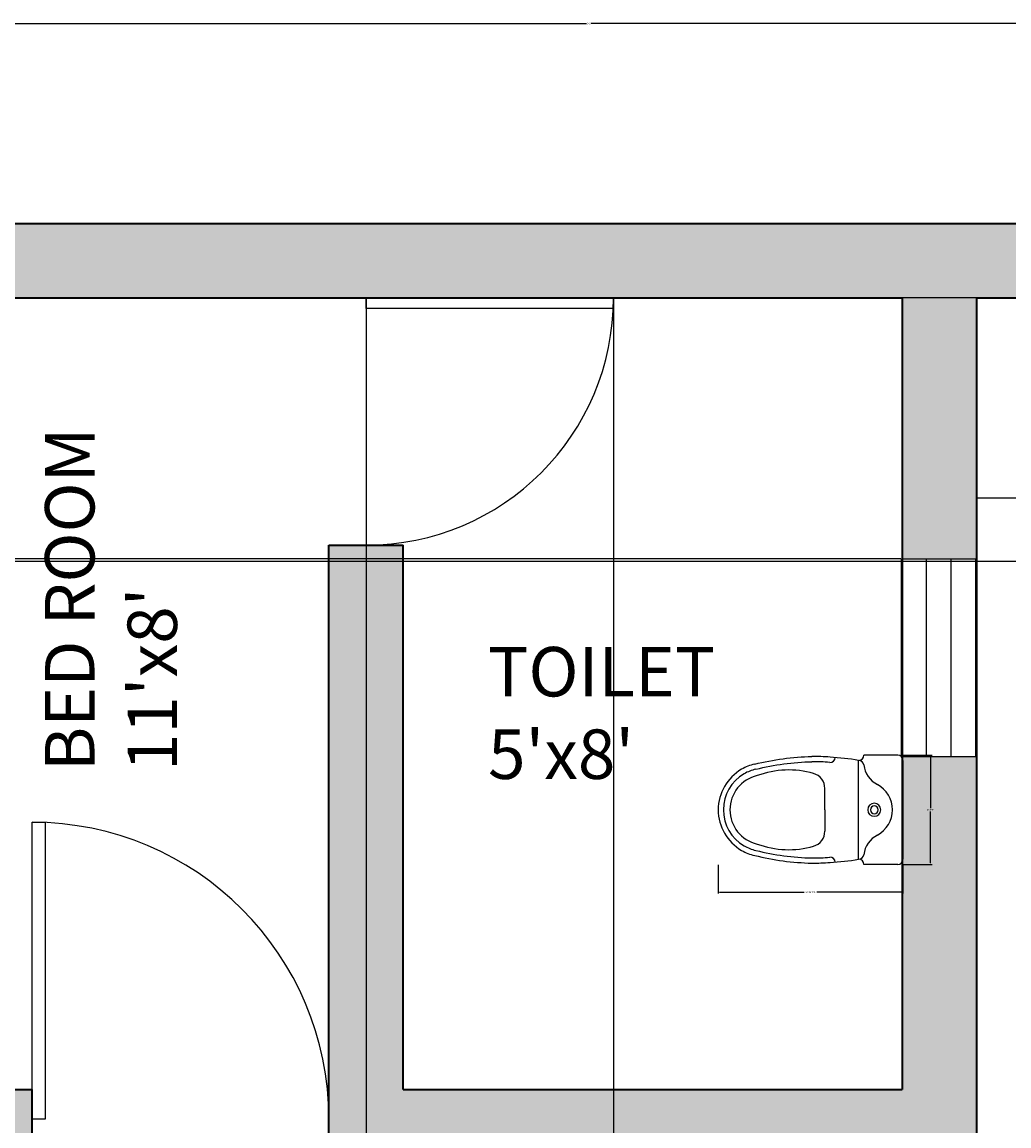
# Model space of a CAD drawing. Units: millimetres. Extents: x 2817 to 5038, y 1110 to 3565.
# Tile 18 of 21: x 2946 to 3065, y 1505 to 1639. Entities that reach past the tile are written whole.
import ezdxf

# ---------------------------------------------------------------- set-up
doc = ezdxf.new("R2010")
doc.units = ezdxf.units.MM
for name, color, linetype, lineweight in [('A-ANNO-DIMS', 2, 'Continuous', 18), ('A-AREA-IDEN', 7, 'Continuous', 18), ('A-FLOR-FIXT', 8, 'Continuous', 18), ('A-WALL', 7, 'Continuous', 35), ('DOOR&WINDOW', 1, 'Continuous', 25)]:
    doc.layers.add(name, color=color, linetype=linetype, lineweight=lineweight)
doc.layers.add('A-WALL-PATT', color=51, linetype='Continuous', lineweight=13, true_color=0xf7f281)
doc.layers.add('THIET-BI', color=21, linetype='Continuous')
doc.styles.get("Standard").update_dxf_attribs({"font": 'arial.ttf'})
doc.dimstyles.get("Standard").update_dxf_attribs({"dimtxt": 0.18, "dimasz": 0.18, "dimexe": 0.18, "dimexo": 0.0625, "dimgap": 0.09, "dimtad": 0, "dimtih": 1, "dimtoh": 1, "dimdec": 4, "dimzin": 0, "dimdsep": 46, "dimtxsty": 'Standard', "dimcen": 0.09, "dimadec": 0, "dimazin": 0, "dimtfac": 1, "dimtdec": 4, "dimtofl": 0, "dimtmove": 0, "dimatfit": 3, "dimfxl": 1, "dimtolj": 1, "dimtzin": 0, "dimarcsym": 0})

# ---------------------------------------------------------------- blocks, each defined once
blk = doc.blocks.new('*U2')
for p, q in [((0, 0), (0, -6)), ((40, 0), (40, -6))]:
    blk.add_line(p, q)
blk.add_lwpolyline([(0, 0), (0, 40), (1.75, 40), (1.75, 0)], close=True)
blk.add_arc((0, 0), 40, 0, 90)
blk = doc.blocks.new('A$C7C314EA1')
at = {"layer": 'THIET-BI'}
for p, q in [((0, 20), (0, 400)), ((20, 420), (150, 420)), ((170, 400), (170, 20)), ((300, 210), (300, 292.2)), ((300, 210), (300, 127.8)), ((20, 0), (150, 0)), ((20, 0), (150, 0))]:
    blk.add_line(p, q, dxfattribs=at)
for points in [[(279.9, 412.5, 0.02753), (170, 400, 0.02753)], [(564.9, 366.1, 0.054905), (349.5, 395, 0.054905)], [(569.7, 385.6, 0.054905), (350, 415, 0.054905)], [(300, 210), (300, 290, 0.704392)], [(300, 210), (300, 130, -0.704392)], [(564.9, 53.9, -0.054905), (349.5, 25, -0.054905)], [(170, 20, 0.02753), (279.9, 7.5, 0.02753)], [(569.7, 34.4, -0.054905), (350, 5, -0.054905)]]:
    blk.add_lwpolyline(points, format="xyb", dxfattribs=at)
for centre, radius, start, end in [((20, 400), 20, 90, 180), ((51, 395.2), 100, 298.1382, 352.7323), ((170, 420), 20, 180, 270), ((170, 380), 20, 90, 172.7323), ((279.9, 412.5), 20, 184.5905, 273.8823), ((350, -585), 1000, 90, 94.0204), ((350, -585), 980, 90, 94.0204), ((530, 210), 180, 60, 77.2425), ((360, 292.2), 60, 105.9249, 180), ((439, 15.2), 348.1, 69.701, 105.9249), ((530, 210), 135, 0, 77.2425), ((530, 210), 160, 60, 77.2425), ((530, 210), 160, 0, 60), ((530, 210), 180, 0, 60), ((150, 210), 110, 118.1382, 180), ((110, 210), 25, 0, 180), ((110, 210), 25, 0, 180), ((110, 210), 15, 0, 180), ((110, 210), 15, 0, 180), ((150, 210), 110, 180, 241.8618), ((150, 210), 110, 180, 241.8618), ((110, 210), 25, 180, 0), ((110, 210), 25, 180, 0), ((110, 210), 15, 180, 0), ((110, 210), 15, 180, 0), ((530, 210), 135, 282.7575, 0), ((530, 210), 160, 300, 0), ((530, 210), 180, 300, 0), ((360, 127.8), 60, 180, 254.0751), ((51, 24.8), 100, 7.2677, 61.8618), ((51, 24.8), 100, 7.2677, 61.8618), ((439, 404.8), 348.1, 254.0751, 290.299), ((530, 210), 160, 282.7575, 300), ((530, 210), 180, 282.7575, 300), ((20, 20), 20, 180, 270), ((170, 0), 20, 90, 180), ((170, 40), 20, 187.2677, 270), ((170, 40), 20, 187.2677, 270), ((279.9, 7.5), 20, 86.1177, 175.4095), ((350, 1005), 1000, 265.9796, 270), ((350, 1005), 980, 265.9796, 270)]:
    blk.add_arc(centre, radius, start, end, dxfattribs=at)
blk = doc.blocks.new('WIN-2FT')
for p, q in [((0, 24), (9, 24)), ((0, 0), (0, 24)), ((3, 24), (3, 0)), ((6, 24), (6, 0)), ((9, 24), (9, 0)), ((9, 0), (0, 0))]:
    blk.add_line(p, q)
blk = doc.blocks.new('*D24')
at = {"layer": 'A-ANNO-DIMS', "color": 0, "lineweight": -2, "transparency": 16777216}
for p, q in [((3029.93, 1536.66), (3029.93, 1533.18)), ((3052.32, 1536.66), (3052.32, 1533.18)), ((3030.11, 1533.36), (3040.35, 1533.36)), ((3052.14, 1533.36), (3041.9, 1533.36))]:
    blk.add_line(p, q, dxfattribs=at)
for points in [[(3030.11, 1533.39), (3030.11, 1533.33), (3029.93, 1533.36)], [(3052.14, 1533.39), (3052.14, 1533.33), (3052.32, 1533.36)]]:
    blk.add_solid(points, dxfattribs=at)
at = {"layer": 'Defpoints', "color": 0, "lineweight": -2, "transparency": 16777216}
for p in [(3029.93, 1536.72), (3052.32, 1536.72), (3029.93, 1533.36)]:
    blk.add_point(p, dxfattribs=at)
at = {"layer": 'A-ANNO-DIMS', "color": 0, "transparency": 16777216, "insert": (3041.13, 1533.36), "char_height": 0.18, "attachment_point": 5}
blk.add_mtext('\\A1;WC 22 TYP.', dxfattribs=at)
blk = doc.blocks.new('*D25')
at = {"layer": 'A-ANNO-DIMS', "color": 0, "lineweight": -2, "transparency": 16777216}
for p, q in [((3052.39, 1549.97), (3055.86, 1549.97)), ((3055.68, 1549.79), (3055.68, 1543.53)), ((3055.68, 1536.9), (3055.68, 1543.16)), ((3052.39, 1536.72), (3055.86, 1536.72))]:
    blk.add_line(p, q, dxfattribs=at)
for points in [[(3055.65, 1549.79), (3055.71, 1549.79), (3055.68, 1549.97)], [(3055.65, 1536.9), (3055.71, 1536.9), (3055.68, 1536.72)]]:
    blk.add_solid(points, dxfattribs=at)
at = {"layer": 'Defpoints', "color": 0, "lineweight": -2, "transparency": 16777216}
for p in [(3052.32, 1549.97), (3052.32, 1536.72), (3055.68, 1536.72)]:
    blk.add_point(p, dxfattribs=at)
at = {"layer": 'A-ANNO-DIMS', "color": 0, "transparency": 16777216, "insert": (3055.68, 1543.35), "char_height": 0.18, "attachment_point": 5}
blk.add_mtext('\\A1;13 TYP.', dxfattribs=at)
blk = doc.blocks.new('*D26')
at = {"layer": 'A-ANNO-DIMS', "color": 0, "lineweight": -2, "transparency": 16777216}
for p, q in [((2841.74, 1614.5), (2841.74, 1638.87)), ((2841.92, 1638.69), (3013.95, 1638.69)), ((3186.56, 1638.69), (3014.53, 1638.69)), ((3186.74, 1614.5), (3186.74, 1638.87))]:
    blk.add_line(p, q, dxfattribs=at)
for points in [[(2841.92, 1638.72), (2841.92, 1638.66), (2841.74, 1638.69)], [(3186.56, 1638.72), (3186.56, 1638.66), (3186.74, 1638.69)]]:
    blk.add_solid(points, dxfattribs=at)
at = {"layer": 'Defpoints', "color": 0, "lineweight": -2, "transparency": 16777216}
for p in [(3186.74, 1638.69), (2841.74, 1614.44), (3186.74, 1614.44)]:
    blk.add_point(p, dxfattribs=at)
at = {"layer": 'A-ANNO-DIMS', "color": 0, "transparency": 16777216, "insert": (3014.24, 1638.69), "char_height": 0.18, "attachment_point": 5}
blk.add_mtext('\\A1;345', dxfattribs=at)
blk = doc.blocks.new('*D35')
at = {"layer": 'A-ANNO-DIMS', "color": 0, "lineweight": -2, "transparency": 16777216}
for p, q in [((2987.24, 1605.37), (2987.24, 1110.01)), ((3017.24, 1605.37), (3017.24, 1110.01)), ((2987.42, 1110.19), (3002.02, 1110.19)), ((3017.06, 1110.19), (3002.46, 1110.19))]:
    blk.add_line(p, q, dxfattribs=at)
for points in [[(2987.42, 1110.22), (2987.42, 1110.16), (2987.24, 1110.19)], [(3017.06, 1110.22), (3017.06, 1110.16), (3017.24, 1110.19)]]:
    blk.add_solid(points, dxfattribs=at)
at = {"layer": 'Defpoints', "color": 0, "lineweight": -2, "transparency": 16777216}
for p in [(2987.24, 1605.44), (3017.24, 1605.44), (3017.24, 1110.19)]:
    blk.add_point(p, dxfattribs=at)
at = {"layer": 'A-ANNO-DIMS', "color": 0, "transparency": 16777216, "insert": (3002.24, 1110.19), "char_height": 0.18, "attachment_point": 5}
blk.add_mtext('\\A1;30', dxfattribs=at)
blk = doc.blocks.new('*D38')
at = {"layer": 'A-ANNO-DIMS', "color": 0, "lineweight": -2, "transparency": 16777216}
for p, q in [((3110.18, 1573.44), (2817.31, 1573.44)), ((2817.49, 1573.26), (2817.49, 1523.62)), ((2817.49, 1473.62), (2817.49, 1523.25)), ((3105.68, 1473.44), (2817.31, 1473.44))]:
    blk.add_line(p, q, dxfattribs=at)
for points in [[(2817.46, 1573.26), (2817.52, 1573.26), (2817.49, 1573.44)], [(2817.46, 1473.62), (2817.52, 1473.62), (2817.49, 1473.44)]]:
    blk.add_solid(points, dxfattribs=at)
at = {"layer": 'Defpoints', "color": 0, "lineweight": -2, "transparency": 16777216}
for p in [(2817.49, 1573.44), (3110.24, 1573.44), (3105.74, 1473.44)]:
    blk.add_point(p, dxfattribs=at)
at = {"layer": 'A-ANNO-DIMS', "color": 0, "transparency": 16777216, "insert": (2817.49, 1523.44), "char_height": 0.18, "attachment_point": 5}
blk.add_mtext('\\A1;100', dxfattribs=at)
blk = doc.blocks.new('*D39')
at = {"layer": 'A-ANNO-DIMS', "color": 0, "lineweight": -2, "transparency": 16777216}
for p, q in [((3105.68, 1605.44), (2817.31, 1605.44)), ((2817.49, 1605.26), (2817.49, 1589.62)), ((2817.49, 1573.62), (2817.49, 1589.25)), ((3110.18, 1573.44), (2817.31, 1573.44))]:
    blk.add_line(p, q, dxfattribs=at)
for points in [[(2817.46, 1605.26), (2817.52, 1605.26), (2817.49, 1605.44)], [(2817.46, 1573.62), (2817.52, 1573.62), (2817.49, 1573.44)]]:
    blk.add_solid(points, dxfattribs=at)
at = {"layer": 'Defpoints', "color": 0, "lineweight": -2, "transparency": 16777216}
for p in [(2817.49, 1605.44), (3105.74, 1605.44), (3110.24, 1573.44)]:
    blk.add_point(p, dxfattribs=at)
at = {"layer": 'A-ANNO-DIMS', "color": 0, "transparency": 16777216, "insert": (2817.49, 1589.44), "char_height": 0.18, "attachment_point": 5}
blk.add_mtext('\\A1;32', dxfattribs=at)
blk = doc.blocks.new('*D41')
at = {"layer": 'A-ANNO-DIMS', "color": 0, "lineweight": -2, "transparency": 16777216}
for p, q in [((3061.24, 1605.37), (3061.24, 1581.01)), ((3105.74, 1605.37), (3105.74, 1581.01)), ((3061.42, 1581.19), (3083.16, 1581.19)), ((3105.56, 1581.19), (3083.82, 1581.19))]:
    blk.add_line(p, q, dxfattribs=at)
for points in [[(3061.42, 1581.22), (3061.42, 1581.16), (3061.24, 1581.19)], [(3105.56, 1581.22), (3105.56, 1581.16), (3105.74, 1581.19)]]:
    blk.add_solid(points, dxfattribs=at)
at = {"layer": 'Defpoints', "color": 0, "lineweight": -2, "transparency": 16777216}
for p in [(3061.24, 1605.44), (3105.74, 1605.44), (3061.24, 1581.19)]:
    blk.add_point(p, dxfattribs=at)
at = {"layer": 'A-ANNO-DIMS', "color": 0, "transparency": 16777216, "insert": (3083.49, 1581.19), "char_height": 0.18, "attachment_point": 5}
blk.add_mtext('\\A1;44.5', dxfattribs=at)
blk = doc.blocks.new('*D46')
at = {"layer": 'A-ANNO-DIMS', "color": 0, "lineweight": -2, "transparency": 16777216}
for p, q in [((3052.18, 1605.44), (2817.31, 1605.44)), ((2817.49, 1605.26), (2817.49, 1589.79)), ((2817.49, 1573.96), (2817.49, 1589.43)), ((3052.08, 1573.78), (2817.31, 1573.78))]:
    blk.add_line(p, q, dxfattribs=at)
for points in [[(2817.46, 1605.26), (2817.52, 1605.26), (2817.49, 1605.44)], [(2817.46, 1573.96), (2817.52, 1573.96), (2817.49, 1573.78)]]:
    blk.add_solid(points, dxfattribs=at)
at = {"layer": 'Defpoints', "color": 0, "lineweight": -2, "transparency": 16777216}
for p in [(2817.49, 1605.44), (3052.24, 1605.44), (3052.14, 1573.78)]:
    blk.add_point(p, dxfattribs=at)
at = {"layer": 'A-ANNO-DIMS', "color": 0, "transparency": 16777216, "insert": (2817.49, 1589.61), "char_height": 0.18, "attachment_point": 5}
blk.add_mtext('\\A1;31.65', dxfattribs=at)

msp = doc.modelspace()

# ---------------------------------------------------------------- hatches: boundary and pattern name
at = {"layer": 'A-WALL-PATT'}
h = msp.add_hatch(color=256, dxfattribs=at)
h.dxf.hatch_style = 1
h.paths.add_polyline_path([(3186.7393, 1614.4357), (2841.7393, 1614.4357), (2841.7393, 1568.614), (2850.7393, 1568.7609), (2850.7393, 1605.4357), (2982.7393, 1605.4357), (2991.7393, 1605.4357), (3052.2393, 1605.4357), (3052.2393, 1573.7835), (3061.2393, 1573.7835), (3061.2393, 1605.4357), (3182.2393, 1605.4357), (3182.2393, 1143.4357), (3181.2393, 1143.4357), (3181.2393, 1134.4357), (3186.7393, 1134.4357)])
h.paths.add_polyline_path([(3061.2393, 1143.4357), (3061.2393, 1147.4357), (3052.2393, 1147.4357), (3052.2393, 1143.4357), (2850.7393, 1143.4357), (2850.7393, 1145.2996), (2841.7393, 1145.2996), (2841.7393, 1134.4357), (3061.2393, 1134.4357)], flags=17)
h.paths.add_polyline_path([(2850.7393, 1265.4357), (2946.7393, 1265.4357), (2946.7393, 1270.8357), (2946.7393, 1274.4357), (2850.7393, 1274.4357), (2850.7381, 1274.4357), (2850.7381, 1274.2564), (2841.7393, 1274.2564), (2841.7393, 1193.1527), (2850.7393, 1193.2996)], flags=17)
h.paths.add_polyline_path([(3061.2393, 1299.098), (3052.2393, 1299.098), (3052.2393, 1274.4357), (2991.7393, 1274.4357), (2991.7393, 1340.4357), (2982.7393, 1340.4357), (2982.7393, 1274.4357), (2982.7393, 1265.4357), (3052.2393, 1265.4357), (3052.2393, 1259.143), (3061.2393, 1259.2899)], flags=17)
h.paths.add_polyline_path([(3061.2393, 1383.4357), (3052.2393, 1383.4357), (3052.2393, 1379.4357), (2931.7393, 1379.4357), (2922.7393, 1379.4357), (2850.7393, 1379.4357), (2850.7381, 1379.4357), (2850.7381, 1379.3646), (2841.7393, 1379.3646), (2841.7393, 1322.1095), (2850.7393, 1322.2564), (2850.7393, 1370.4357), (2982.7393, 1370.4357), (2987.2393, 1370.4357), (3017.2393, 1370.4357), (3052.2393, 1370.4357), (3052.2393, 1323.098), (3061.2393, 1323.098)], flags=17)
h = msp.add_hatch(color=256, dxfattribs=at)
h.dxf.hatch_style = 1
h.paths.add_polyline_path([(3061.2393, 1549.7835), (3052.2393, 1549.7835), (3052.2393, 1509.4357), (2991.7393, 1509.4357), (2991.7393, 1575.4357), (2982.7393, 1575.4357), (2982.7393, 1509.4357), (2982.7393, 1500.4357), (3052.2393, 1500.4357), (3052.2393, 1498.4661), (3061.2393, 1498.613)])
h.paths.add_polyline_path([(2946.7393, 1505.8357), (2946.7393, 1509.4357), (2850.7393, 1509.4357), (2850.7393, 1520.7609), (2841.7393, 1520.7609), (2841.7393, 1427.2177), (2850.7393, 1427.3646), (2850.7393, 1500.4357), (2922.7393, 1500.4357), (2931.7393, 1500.4357), (2946.7393, 1500.4357)])
h.paths.add_polyline_path([(3061.2393, 1450.613), (3052.2393, 1450.613), (3052.2393, 1431.4357), (3059.4393, 1431.4357), (3061.2393, 1431.4357)])
h.paths.add_polyline_path([(3061.2393, 1211.2899), (3052.2393, 1211.2899), (3052.2393, 1195.4357), (3059.4393, 1195.4357), (3061.2393, 1195.4357)])

# ---------------------------------------------------------------- linework, layer by layer
at = {"layer": 'A-WALL'}
for p, q in [((2841.7393, 1614.4357), (3186.7393, 1614.4357)), ((2850.7393, 1605.4357), (2982.7393, 1605.4357)), ((2982.7393, 1605.4357), (2991.7393, 1605.4357)), ((2991.7393, 1605.4357), (3052.2393, 1605.4357)), ((3052.2393, 1605.4357), (3052.2393, 1509.4357)), ((3061.2393, 1605.4357), (3061.2393, 1509.4357)), ((3061.2393, 1605.4357), (3182.2393, 1605.4357)), ((3061.2393, 1605.4357), (3061.2393, 1431.4357)), ((2982.7393, 1509.4357), (2982.7393, 1575.4357)), ((2982.7393, 1509.4357), (2982.7393, 1575.4357)), ((2982.7393, 1575.4357), (2991.7393, 1575.4357)), ((2991.7393, 1509.4357), (2991.7393, 1575.4357)), ((2850.7393, 1509.4357), (2946.7393, 1509.4357)), ((2946.7393, 1500.4357), (2946.7393, 1509.4357)), ((2982.7393, 1500.4357), (2982.7393, 1509.4357)), ((2991.7393, 1509.4357), (3052.2393, 1509.4357))]:
    msp.add_line(p, q, dxfattribs=at)

# ---------------------------------------------------------------- block references
at = {"layer": 'A-FLOR-FIXT', "xscale": 0.0315352998736587, "yscale": 0.0315352998736587, "zscale": 0.0315352998736587, "rotation": 180}
msp.add_blockref('A$C7C314EA1', (3052.3225, 1549.9682), dxfattribs=at)
at = {"layer": 'DOOR&WINDOW', "xscale": 0.75, "yscale": 0.75, "zscale": 0.75, "rotation": 270}
msp.add_blockref('*U2', (2987.2393, 1605.4357), dxfattribs=at)
at = {"layer": 'DOOR&WINDOW'}
msp.add_blockref('WIN-2FT', (3052.1378, 1549.7835), dxfattribs=at)
at = {"layer": 'DOOR&WINDOW', "xscale": 0.9, "yscale": 0.9, "zscale": 0.9}
msp.add_blockref('*U2', (2946.7393, 1505.8357), dxfattribs=at)

# ---------------------------------------------------------------- texts
at = {"layer": 'A-AREA-IDEN', "insert": (2948.3143, 1548.0447), "char_height": 6, "attachment_point": 1, "rotation": 90}
msp.add_mtext_dynamic_manual_height_columns("BED ROOM\\P11'x8'", width=48.483628, gutter_width=12.5, heights=[0], dxfattribs=at)
at = {"layer": 'A-AREA-IDEN', "insert": (3002.0276, 1563.0922), "char_height": 6, "attachment_point": 1}
msp.add_mtext_dynamic_manual_height_columns("TOILET\\P5'x8'", width=42.068425, gutter_width=12.5, heights=[0], dxfattribs=at)

# ---------------------------------------------------------------- dimensions: what is measured, and where the dimension line sits
at = {"layer": 'A-ANNO-DIMS'}
for base, p1, p2, picture, middle in [((3186.7393, 1638.6857), (2841.7393, 1614.4357), (3186.7393, 1614.4357), '*D26', (3014.2393, 1638.6857)), ((3017.2393, 1110.1857), (2987.2393, 1605.4357), (3017.2393, 1605.4357), '*D35', (3002.2393, 1110.1857))]:
    dim = msp.add_linear_dim(base=base, p1=p1, p2=p2, dimstyle='Standard', override={"dimdec": 0, "dimlfac": 1, "dimrnd": 0, "dimzin": 0, "dimdsep": 46, "dimlunit": 2}, dxfattribs=at)
    dim.commit()
    dim.dimension.update_dxf_attribs({"geometry": picture, "text_midpoint": middle})
for base, p1, p2, angle, override, picture, middle in [((2817.4881, 1605.4357), (3052.1378, 1573.7835), (3052.2393, 1605.4357), 90, {"dimdec": 2, "dimlfac": 1, "dimrnd": 0, "dimzin": 0, "dimdsep": 46, "dimlunit": 2}, '*D46', (2817.4881, 1589.6096)), ((2817.4881, 1605.4357), (3110.2393, 1573.4357), (3105.7393, 1605.4357), 90, {"dimdec": 0, "dimlfac": 1, "dimrnd": 0, "dimzin": 0, "dimdsep": 46, "dimlunit": 2}, '*D39', (2817.4881, 1589.4357)), ((3061.2393, 1581.1857), (3105.7393, 1605.4357), (3061.2393, 1605.4357), 180, {"dimdec": 1, "dimlfac": 1, "dimrnd": 0, "dimzin": 0, "dimdsep": 46, "dimlunit": 2}, '*D41', (3083.4893, 1581.1857)), ((2817.4881, 1573.4357), (3105.7393, 1473.4357), (3110.2393, 1573.4357), 90, {"dimdec": 0, "dimlfac": 1, "dimrnd": 0, "dimzin": 0, "dimdsep": 46, "dimlunit": 2}, '*D38', (2817.4881, 1523.4357))]:
    dim = msp.add_linear_dim(base=base, p1=p1, p2=p2, angle=angle, dimstyle='Standard', override=override, dxfattribs=at)
    dim.commit()
    dim.dimension.update_dxf_attribs({"geometry": picture, "text_midpoint": middle})
for base, p1, p2, angle, text, picture, middle in [((3055.681, 1536.7234), (3052.3225, 1549.9682), (3052.3225, 1536.7234), 270, '<> TYP.', '*D25', (3055.681, 1543.3458)), ((3029.9324, 1533.3649), (3052.3225, 1536.7234), (3029.9324, 1536.7234), 180, 'WC <> TYP.', '*D24', (3041.1275, 1533.3649))]:
    dim = msp.add_linear_dim(base=base, p1=p1, p2=p2, angle=angle, text=text, dimstyle='Standard', override={"dimdec": 0, "dimlfac": 1, "dimrnd": 0, "dimzin": 0, "dimdsep": 46, "dimlunit": 2}, dxfattribs=at)
    dim.commit()
    dim.dimension.update_dxf_attribs({"geometry": picture, "text_midpoint": middle})

doc.saveas('drawing.dxf')
